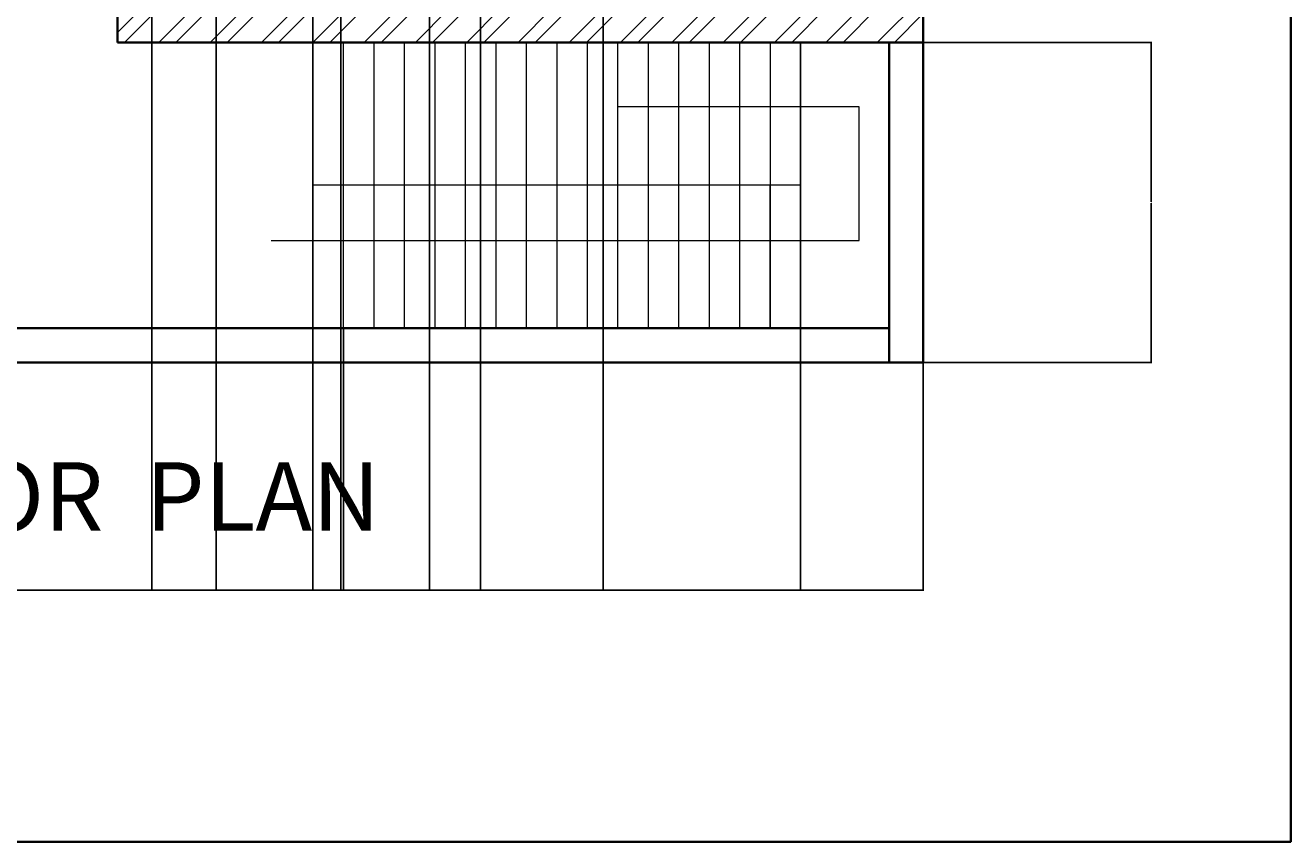
# Model space of a CAD drawing. Units: inches. Extents: x 2552 to 3217, y 1417 to 2737.
# Tile 4 of 25: x 2885 to 3217, y 1417 to 1631. Entities that reach past the tile are written whole.
import ezdxf

# ---------------------------------------------------------------- set-up
doc = ezdxf.new("R2010")
doc.units = ezdxf.units.IN
for name, color, linetype, lineweight in [('A-ANNO-DIMS', 2, 'Continuous', 18), ('A-ANNO-TEXT', 7, 'Continuous', 25), ('A-ANNO-TTLB', 7, 'Continuous', 35), ('A-FLOR-STRS', 140, 'Continuous', 20), ('A-WALL', 7, 'Continuous', 35), ('A-WALL-PATT', 217, 'Continuous', 13)]:
    doc.layers.add(name, color=color, linetype=linetype, lineweight=lineweight)
doc.styles.get("Standard").update_dxf_attribs({"font": 'arial.ttf'})
doc.dimstyles.get("Standard").update_dxf_attribs({"dimtxt": 0.18, "dimasz": 0.18, "dimexe": 0.18, "dimexo": 0.0625, "dimgap": 0.09, "dimtad": 0, "dimtih": 1, "dimtoh": 1, "dimdec": 4, "dimzin": 0, "dimdsep": 46, "dimtxsty": 'Standard', "dimcen": 0.09, "dimadec": 0, "dimazin": 0, "dimtfac": 1, "dimtdec": 4, "dimtofl": 0, "dimtmove": 0, "dimatfit": 3, "dimfxl": 1, "dimtolj": 1, "dimtzin": 0, "dimarcsym": 0})

# ---------------------------------------------------------------- blocks, each defined once
blk = doc.blocks.new('*D49')
at = {"layer": 'A-ANNO-DIMS', "color": 0, "lineweight": -2, "transparency": 16777216}
for p, q in [((2637.35, 1542.45), (2637.35, 1482.53)), ((3120.35, 1542.45), (3120.35, 1482.53)), ((2637.53, 1482.71), (2878.56, 1482.71)), ((3120.17, 1482.71), (2879.15, 1482.71))]:
    blk.add_line(p, q, dxfattribs=at)
at = {"layer": 'A-ANNO-DIMS', "color": 0, "transparency": 16777216}
for points in [[(2637.53, 1482.74), (2637.53, 1482.68), (2637.35, 1482.71)], [(3120.17, 1482.74), (3120.17, 1482.68), (3120.35, 1482.71)]]:
    blk.add_solid(points, dxfattribs=at)
at = {"layer": 'Defpoints', "color": 0, "transparency": 16777216}
for p in [(2637.35, 1542.51), (3120.35, 1542.51), (3120.35, 1482.71)]:
    blk.add_point(p, dxfattribs=at)
at = {"layer": 'A-ANNO-DIMS', "color": 0, "transparency": 16777216, "insert": (2878.85, 1482.71), "char_height": 0.18, "attachment_point": 5}
blk.add_mtext('\\A1;483', dxfattribs=at)
blk = doc.blocks.new('*D53')
at = {"layer": 'A-ANNO-DIMS', "color": 0, "lineweight": -2, "transparency": 16777216}
for p, q in [((3120.42, 1626.51), (3180.33, 1626.51)), ((3180.15, 1626.33), (3180.15, 1584.69)), ((3180.15, 1542.69), (3180.15, 1584.33)), ((3120.42, 1542.51), (3180.33, 1542.51))]:
    blk.add_line(p, q, dxfattribs=at)
at = {"layer": 'A-ANNO-DIMS', "color": 0, "transparency": 16777216}
for points in [[(3180.12, 1626.33), (3180.18, 1626.33), (3180.15, 1626.51)], [(3180.12, 1542.69), (3180.18, 1542.69), (3180.15, 1542.51)]]:
    blk.add_solid(points, dxfattribs=at)
at = {"layer": 'Defpoints', "color": 0, "transparency": 16777216}
for p in [(3120.35, 1626.51), (3180.15, 1626.51), (3120.35, 1542.51)]:
    blk.add_point(p, dxfattribs=at)
at = {"layer": 'A-ANNO-DIMS', "color": 0, "transparency": 16777216, "insert": (3180.15, 1584.51), "char_height": 0.18, "attachment_point": 5}
blk.add_mtext('\\A1;84', dxfattribs=at)
blk = doc.blocks.new('*D56')
at = {"layer": 'A-ANNO-DIMS', "color": 0, "lineweight": -2, "transparency": 16777216}
for p, q in [((2967.49, 2515.95), (2967.49, 1482.53)), ((2990.69, 2515.95), (2990.69, 1482.53)), ((2967.67, 1482.71), (2978.76, 1482.71)), ((2990.51, 1482.71), (2979.41, 1482.71))]:
    blk.add_line(p, q, dxfattribs=at)
at = {"layer": 'A-ANNO-DIMS', "color": 0, "transparency": 16777216}
for points in [[(2967.67, 1482.74), (2967.67, 1482.68), (2967.49, 1482.71)], [(2990.51, 1482.74), (2990.51, 1482.68), (2990.69, 1482.71)]]:
    blk.add_solid(points, dxfattribs=at)
at = {"layer": 'Defpoints', "color": 0, "transparency": 16777216}
for p in [(2967.49, 2516.01), (2990.69, 2516.01), (2990.69, 1482.71)]:
    blk.add_point(p, dxfattribs=at)
at = {"layer": 'A-ANNO-DIMS', "color": 0, "transparency": 16777216, "insert": (2979.09, 1482.71), "char_height": 0.18, "attachment_point": 5}
blk.add_mtext('\\A1;23.2', dxfattribs=at)
blk = doc.blocks.new('*D57')
at = {"layer": 'A-ANNO-DIMS', "color": 0, "lineweight": -2, "transparency": 16777216}
for p, q in [((3004.08, 2515.95), (3004.08, 1482.53)), ((3036.34, 2515.95), (3036.34, 1482.53)), ((3004.26, 1482.71), (3019.75, 1482.71)), ((3036.16, 1482.71), (3020.68, 1482.71))]:
    blk.add_line(p, q, dxfattribs=at)
at = {"layer": 'A-ANNO-DIMS', "color": 0, "transparency": 16777216}
for points in [[(3004.26, 1482.74), (3004.26, 1482.68), (3004.08, 1482.71)], [(3036.16, 1482.74), (3036.16, 1482.68), (3036.34, 1482.71)]]:
    blk.add_solid(points, dxfattribs=at)
at = {"layer": 'Defpoints', "color": 0, "transparency": 16777216}
for p in [(3004.08, 2516.01), (3036.34, 2516.01), (3036.34, 1482.71)]:
    blk.add_point(p, dxfattribs=at)
at = {"layer": 'A-ANNO-DIMS', "color": 0, "transparency": 16777216, "insert": (3020.21, 1482.71), "char_height": 0.18, "attachment_point": 5}
blk.add_mtext('\\A1;32.255', dxfattribs=at)
blk = doc.blocks.new('*D62')
at = {"layer": 'A-ANNO-DIMS', "color": 0, "lineweight": -2, "transparency": 16777216}
for p, q in [((2960.11, 1626.45), (2960.11, 1482.53)), ((3088.11, 1626.45), (3088.11, 1482.53)), ((2960.29, 1482.71), (3023.83, 1482.71)), ((3087.93, 1482.71), (3024.39, 1482.71))]:
    blk.add_line(p, q, dxfattribs=at)
at = {"layer": 'A-ANNO-DIMS', "color": 0, "transparency": 16777216}
for points in [[(2960.29, 1482.74), (2960.29, 1482.68), (2960.11, 1482.71)], [(3087.93, 1482.74), (3087.93, 1482.68), (3088.11, 1482.71)]]:
    blk.add_solid(points, dxfattribs=at)
at = {"layer": 'Defpoints', "color": 0, "transparency": 16777216}
for p in [(2960.11, 1626.51), (3088.11, 1626.51), (3088.11, 1482.71)]:
    blk.add_point(p, dxfattribs=at)
at = {"layer": 'A-ANNO-DIMS', "color": 0, "transparency": 16777216, "insert": (3024.11, 1482.71), "char_height": 0.18, "attachment_point": 5}
blk.add_mtext('\\A1;128', dxfattribs=at)
blk = doc.blocks.new('*D63')
at = {"layer": 'A-ANNO-DIMS', "color": 0, "lineweight": -2, "transparency": 16777216}
for p, q in [((2960.11, 1551.45), (2960.11, 1482.53)), ((2968.11, 1551.45), (2968.11, 1482.53)), ((2960.29, 1482.71), (2963.96, 1482.71)), ((2967.93, 1482.71), (2964.26, 1482.71))]:
    blk.add_line(p, q, dxfattribs=at)
at = {"layer": 'A-ANNO-DIMS', "color": 0, "transparency": 16777216}
for points in [[(2960.29, 1482.74), (2960.29, 1482.68), (2960.11, 1482.71)], [(2967.93, 1482.74), (2967.93, 1482.68), (2968.11, 1482.71)]]:
    blk.add_solid(points, dxfattribs=at)
at = {"layer": 'Defpoints', "color": 0, "transparency": 16777216}
for p in [(2960.11, 1551.51), (2968.11, 1551.51), (2968.11, 1482.71)]:
    blk.add_point(p, dxfattribs=at)
at = {"layer": 'A-ANNO-DIMS', "color": 0, "transparency": 16777216, "insert": (2964.11, 1482.71), "char_height": 0.18, "attachment_point": 5}
blk.add_mtext('\\A1;8', dxfattribs=at)
blk = doc.blocks.new('*D64')
at = {"layer": 'A-ANNO-DIMS', "color": 0, "lineweight": -2, "transparency": 16777216}
for p, q in [((2646.35, 1551.58), (2646.35, 2709.49)), ((2646.53, 2709.31), (2802.77, 2709.31)), ((2959.93, 2709.31), (2803.69, 2709.31)), ((2960.11, 1551.58), (2960.11, 2709.49))]:
    blk.add_line(p, q, dxfattribs=at)
at = {"layer": 'A-ANNO-DIMS', "color": 0, "transparency": 16777216}
for points in [[(2646.53, 2709.34), (2646.53, 2709.28), (2646.35, 2709.31)], [(2959.93, 2709.34), (2959.93, 2709.28), (2960.11, 2709.31)]]:
    blk.add_solid(points, dxfattribs=at)
at = {"layer": 'Defpoints', "color": 0, "transparency": 16777216}
for p in [(2960.11, 2709.31), (2646.35, 1551.51), (2960.11, 1551.51)]:
    blk.add_point(p, dxfattribs=at)
at = {"layer": 'A-ANNO-DIMS', "color": 0, "transparency": 16777216, "insert": (2803.23, 2709.31), "char_height": 0.18, "attachment_point": 5}
blk.add_mtext('\\A1;313.76', dxfattribs=at)
blk = doc.blocks.new('*D67')
at = {"layer": 'A-ANNO-DIMS', "color": 0, "lineweight": -2, "transparency": 16777216}
for p, q in [((2917.85, 2640.45), (2917.85, 1482.53)), ((2934.77, 2624.73), (2934.77, 1482.53)), ((2918.03, 1482.71), (2925.86, 1482.71)), ((2934.59, 1482.71), (2926.76, 1482.71))]:
    blk.add_line(p, q, dxfattribs=at)
at = {"layer": 'A-ANNO-DIMS', "color": 0, "transparency": 16777216}
for points in [[(2918.03, 1482.74), (2918.03, 1482.68), (2917.85, 1482.71)], [(2934.59, 1482.74), (2934.59, 1482.68), (2934.77, 1482.71)]]:
    blk.add_solid(points, dxfattribs=at)
at = {"layer": 'Defpoints', "color": 0, "transparency": 16777216}
for p in [(2917.85, 2640.51), (2934.77, 2624.79), (2934.77, 1482.71)]:
    blk.add_point(p, dxfattribs=at)
at = {"layer": 'A-ANNO-DIMS', "color": 0, "transparency": 16777216, "insert": (2926.31, 1482.71), "char_height": 0.18, "attachment_point": 5}
blk.add_mtext('\\A1;16.912', dxfattribs=at)

msp = doc.modelspace()

# ---------------------------------------------------------------- hatches: boundary and pattern name
at = {"layer": 'A-WALL-PATT'}
h = msp.add_hatch(dxfattribs=at)
h.set_pattern_fill('ANSI32', color=256)
h.paths.add_polyline_path([(2756.676, 2649.5125), (2637.3535, 2649.5125), (2637.3535, 2617.9626), (2641.8535, 2617.9626), (2646.3535, 2617.9626), (2646.3535, 2640.5125), (2724.3535, 2640.5125), (2724.3535, 2520.5125), (2720.299, 2520.5125), (2720.299, 2516.0125), (2733.4075, 2516.0125), (2733.4075, 2518.2213), (2733.4075, 2520.5125), (2728.8535, 2520.5125), (2728.8535, 2640.5125), (2756.676, 2640.5125)])
h.paths.add_polyline_path([(2848.8535, 2649.5125), (2804.676, 2649.5125), (2804.676, 2640.5125), (2839.8535, 2640.5125), (2839.8535, 2598.3517), (2848.8535, 2598.3517)])
h.paths.add_polyline_path([(2646.3535, 2516.0125), (2697.9593, 2516.0125), (2697.9593, 2518.2625), (2697.9593, 2520.5125), (2646.3535, 2520.5125), (2646.3535, 2581.9626), (2637.3535, 2581.9626), (2637.3535, 2364.3298), (2646.3535, 2364.3298), (2646.3535, 2387.0125), (2724.3535, 2387.0125), (2724.3535, 2267.0125), (2721.0443, 2267.0125), (2721.0443, 2262.5125), (2733.7854, 2262.5125), (2733.7854, 2264.7625), (2733.7854, 2267.0125), (2728.8535, 2267.0125), (2728.8535, 2387.0125), (2839.8535, 2387.0125), (2839.8535, 2363.8387), (2848.8535, 2363.8387), (2848.8535, 2403.7415), (2844.3535, 2403.7415), (2839.8535, 2403.7415), (2839.8535, 2396.0125), (2646.3535, 2396.0125)])
h.paths.add_polyline_path([(2848.8535, 2550.3517), (2844.3535, 2550.3517), (2839.8535, 2550.3517), (2839.8535, 2520.5125), (2801.9195, 2520.5125), (2801.9195, 2518.2625), (2801.9195, 2516.0125), (2839.8535, 2516.0125), (2839.8535, 2507.5813), (2848.8535, 2507.5813)], flags=17)
h.paths.add_polyline_path([(2848.8535, 2483.5813), (2844.3535, 2483.5813), (2839.8535, 2483.5813), (2839.8535, 2468.0125), (2773.8535, 2468.0125), (2773.8535, 2516.0125), (2778.1336, 2516.0125), (2778.1336, 2520.5125), (2766.696, 2520.5125), (2766.696, 2518.2625), (2766.696, 2516.0125), (2769.3535, 2516.0125), (2769.3535, 2463.5125), (2839.8535, 2463.5125), (2839.8535, 2431.0782), (2848.8535, 2431.0782)], flags=17)
h.paths.add_polyline_path([(2917.8535, 2569.2764), (2913.3535, 2569.2764), (2908.8535, 2569.2764), (2908.8535, 2433.001), (2917.8535, 2433.001), (2917.8535, 2516.0125), (2967.486, 2516.0125), (2967.486, 2520.5125), (2917.8535, 2520.5125)])
h.paths.add_polyline_path([(3000.3535, 2640.5125), (2995.8535, 2640.5125), (2995.8535, 2520.5125), (2990.688, 2520.5125), (2990.688, 2516.0125), (3004.0844, 2516.0125), (3004.0844, 2518.2625), (3004.0844, 2520.5125), (3000.3535, 2520.5125)])
h.paths.add_polyline_path([(3120.3535, 2561.3689), (3115.8535, 2561.3689), (3111.3535, 2561.3689), (3111.3535, 2520.5125), (3070.9814, 2520.5125), (3070.9814, 2518.2625), (3070.9814, 2516.0125), (3111.3535, 2516.0125), (3111.3535, 2505.1841), (3120.3535, 2505.1841)])
h.paths.add_polyline_path([(3120.3535, 2481.1841), (3115.8535, 2481.1841), (3111.3535, 2481.1841), (3111.3535, 2468.0125), (3045.3535, 2468.0125), (3045.3535, 2516.0125), (3048.9787, 2516.0125), (3048.9787, 2520.5125), (3036.3395, 2520.5125), (3036.3395, 2516.0125), (3040.8535, 2516.0125), (3040.8535, 2463.5125), (3111.3535, 2463.5125), (3111.3535, 2396.0125), (2917.8535, 2396.0125), (2917.8535, 2403.4124), (2913.3535, 2403.4124), (2908.8535, 2403.4124), (2908.8535, 2182.5756), (2917.8535, 2182.5756), (2917.8535, 2262.5125), (2968.001, 2262.5125), (2968.001, 2264.7625), (2968.001, 2267.0125), (2917.8535, 2267.0125), (2917.8535, 2387.0125), (3111.3535, 2387.0125), (3111.3535, 2352.2435), (3120.3535, 2352.2435)])
h.paths.add_polyline_path([(3120.3535, 2304.2435), (3115.8535, 2304.2435), (3111.3535, 2304.2435), (3111.3535, 2267.0125), (3073.8616, 2267.0125), (3073.8616, 2264.7625), (3073.8616, 2262.5125), (3111.3535, 2262.5125), (3111.3535, 2252.376), (3120.3535, 2252.376)], flags=17)
h.paths.add_polyline_path([(3120.3535, 2228.376), (3115.8535, 2228.376), (3111.3535, 2228.376), (3111.3535, 2214.5125), (3045.3535, 2214.5125), (3045.3535, 2262.5125), (3049.3096, 2262.5125), (3049.3096, 2267.0125), (3035.0125, 2267.0125), (3035.0125, 2262.5125), (3040.8535, 2262.5125), (3040.8535, 2210.0125), (3111.3535, 2210.0125), (3111.3535, 2142.5125), (2917.8535, 2142.5125), (2917.8535, 2150.2408), (2913.3535, 2150.2408), (2908.8535, 2150.2408), (2908.8535, 1924.9905), (2917.8535, 1924.9905), (2917.8535, 2009.0125), (2971.959, 2009.0125), (2971.959, 2011.2625), (2971.959, 2013.5125), (2917.8535, 2013.5125), (2917.8535, 2133.5125), (2995.8535, 2133.5125), (2995.8535, 2013.5125), (2992.1797, 2013.5125), (2992.1797, 2009.0125), (3004.3344, 2009.0125), (3004.3344, 2011.2625), (3004.3344, 2013.5125), (3000.3535, 2013.5125), (3000.3535, 2133.5125), (3111.3535, 2133.5125), (3111.3535, 2115.0291), (3120.3535, 2115.0291)])
h.paths.add_polyline_path([(3000.3535, 2387.0125), (2995.8535, 2387.0125), (2995.8535, 2267.0125), (2991.3326, 2267.0125), (2991.3326, 2262.5125), (3004.1044, 2262.5125), (3004.1044, 2264.7625), (3004.1044, 2267.0125), (3000.3535, 2267.0125)], flags=17)
h.paths.add_polyline_path([(3120.3535, 1973.2388), (3115.8535, 1973.2388), (3111.3535, 1973.2388), (3111.3535, 1961.0125), (3045.3535, 1961.0125), (3045.3535, 2009.0125), (3048.9101, 2009.0125), (3048.9101, 2013.5125), (3037.105, 2013.5125), (3037.105, 2011.2625), (3037.105, 2009.0125), (3040.8535, 2009.0125), (3040.8535, 1956.5125), (3111.3535, 1956.5125), (3111.3535, 1889.0125), (2917.8535, 1889.0125), (2917.8535, 1895.7215), (2913.3535, 1895.7215), (2908.8535, 1895.7215), (2908.8535, 1844.2217), (2917.8535, 1844.2217), (2917.8535, 1880.0125), (3111.3535, 1880.0125), (3111.3535, 1846.9541), (3120.3535, 1846.9541)])
h.paths.add_polyline_path([(3120.3535, 2067.0291), (3111.3535, 2067.0291), (3111.3535, 2013.5125), (3071.3001, 2013.5125), (3071.3001, 2009.0125), (3111.3535, 2009.0125), (3111.3535, 1997.2388), (3120.3535, 1997.2388)], flags=0)
h.paths.add_polyline_path([(3120.3535, 1798.9541), (3115.8535, 1798.9541), (3111.3535, 1798.9541), (3111.3535, 1760.0125), (3071.2497, 1760.0125), (3071.2497, 1757.7625), (3071.2497, 1755.5125), (3111.3535, 1755.5125), (3111.3535, 1746.162), (3120.3535, 1746.2478)])
h.paths.add_polyline_path([(3120.3535, 1722.2049), (3111.3535, 1722.2049), (3111.3535, 1707.5125), (3045.3535, 1707.5125), (3045.3535, 1755.5125), (3048.6624, 1755.5125), (3048.6624, 1760.0125), (3035.3703, 1760.0125), (3035.3703, 1755.5125), (3040.8535, 1755.5125), (3040.8535, 1703.0125), (3111.3535, 1703.0125), (3111.3535, 1635.5125), (2917.8535, 1635.5125), (2917.8535, 1643.1366), (2913.3535, 1643.1366), (2908.8535, 1643.1366), (2908.8535, 1626.5125), (3120.3535, 1626.5125)])
h.paths.add_polyline_path([(2917.8535, 1755.5125), (2973.2287, 1755.5125), (2973.2287, 1757.7625), (2973.2287, 1760.0125), (2917.8535, 1760.0125), (2917.8535, 1808.2217), (2913.3535, 1808.2217), (2908.8535, 1808.2217), (2908.8535, 1676.1665), (2917.8535, 1676.1665)])
h.paths.add_polyline_path([(3000.3535, 1880.0125), (2995.8535, 1880.0125), (2995.8535, 1760.0125), (2992.9329, 1760.0125), (2992.9329, 1755.5125), (3003.8766, 1755.5125), (3003.8766, 1757.7625), (3003.8766, 1760.0125), (3000.3535, 1760.0125)])
h.paths.add_polyline_path([(2848.8535, 1896.6971), (2844.3535, 1896.6971), (2839.8535, 1896.6971), (2839.8535, 1889.0125), (2646.3535, 1889.0125), (2646.3535, 2009.0125), (2700.5253, 2009.0125), (2700.5253, 2011.2625), (2700.5253, 2013.5125), (2646.3535, 2013.5125), (2646.3535, 2053.1812), (2641.8535, 2053.1812), (2637.3535, 2053.1812), (2637.3535, 1836.254), (2646.3535, 1836.254), (2646.3535, 1880.0125), (2724.3535, 1880.0125), (2724.3535, 1760.0125), (2721.2473, 1760.0125), (2721.2473, 1755.5125), (2731.9187, 1755.5125), (2731.9187, 1757.7625), (2731.9187, 1760.0125), (2728.8535, 1760.0125), (2728.8535, 1880.0125), (2839.8535, 1880.0125), (2839.8535, 1840.3813), (2848.8535, 1840.3813)])
h.paths.add_polyline_path([(2848.8535, 1792.3813), (2844.3535, 1792.3813), (2839.8535, 1792.3813), (2839.8535, 1760.0125), (2797.8845, 1760.0125), (2797.8845, 1755.5125), (2839.8535, 1755.5125), (2839.8535, 1743.3688), (2844.3535, 1743.3688), (2848.8535, 1743.3688)], flags=0)
h.paths.add_polyline_path([(2848.8535, 1719.3688), (2844.3535, 1719.3688), (2839.8535, 1719.3688), (2839.8535, 1707.5125), (2773.8535, 1707.5125), (2773.8535, 1755.5125), (2777.716, 1755.5125), (2777.716, 1760.0125), (2760.9247, 1760.0125), (2760.9247, 1757.9721), (2760.9247, 1755.5125), (2769.3535, 1755.5125), (2769.3535, 1703.0125), (2839.8535, 1703.0125), (2839.8535, 1673.0277), (2848.8535, 1672.9407)], flags=0)
h.paths.add_polyline_path([(2646.3535, 1755.5125), (2702.9171, 1755.5125), (2702.9171, 1757.7625), (2702.9171, 1760.0125), (2646.3535, 1760.0125), (2646.3535, 1800.254), (2641.8535, 1800.254), (2637.3535, 1800.254), (2637.3535, 1626.5125), (2848.8535, 1626.5125), (2848.8535, 1643.1187), (2844.3535, 1643.1187), (2839.8535, 1643.1187), (2839.8535, 1635.5125), (2646.3535, 1635.5125)])
h.paths.add_polyline_path([(2848.8535, 2148.8427), (2844.3535, 2148.8427), (2839.8535, 2148.8427), (2839.8535, 2142.5125), (2646.3535, 2142.5125), (2646.3535, 2262.5125), (2701.3562, 2262.5125), (2701.3562, 2264.7625), (2701.3562, 2267.0125), (2646.3535, 2267.0125), (2646.3535, 2328.3298), (2637.3535, 2328.3298), (2637.3535, 2089.1812), (2646.3535, 2089.1812), (2646.3535, 2133.5125), (2839.8535, 2133.5125), (2839.8535, 2097.5966), (2848.8535, 2097.5966)])
h.paths.add_polyline_path([(2728.8535, 2133.5125), (2724.3535, 2133.5125), (2724.3535, 2013.5125), (2719.6039, 2013.5125), (2719.6039, 2009.0125), (2732.5784, 2009.0125), (2732.5784, 2011.2625), (2732.5784, 2013.5125), (2728.8535, 2013.5125)])
h.paths.add_polyline_path([(2848.8535, 1970.0557), (2844.3535, 1970.0557), (2839.8535, 1970.0557), (2839.8535, 1961.0125), (2773.8535, 1961.0125), (2773.8535, 2009.0125), (2777.3388, 2009.0125), (2777.3388, 2013.5125), (2764.7681, 2013.5125), (2764.7681, 2009.0125), (2769.3535, 2009.0125), (2769.3535, 1956.5125), (2839.8535, 1956.5125), (2839.8535, 1924.7199), (2848.8535, 1924.7199)], flags=17)
h.paths.add_polyline_path([(2848.8535, 2049.5966), (2844.3535, 2049.5966), (2839.8535, 2049.5966), (2839.8535, 2013.5125), (2798.198, 2013.5125), (2798.198, 2011.2625), (2798.198, 2009.0125), (2839.8535, 2009.0125), (2839.8535, 1994.0557), (2848.8535, 1994.0557)], flags=17)
h.paths.add_polyline_path([(2848.8535, 2315.8387), (2839.8535, 2315.8387), (2839.8535, 2267.0125), (2799.3375, 2267.0125), (2799.3375, 2264.7625), (2799.3375, 2262.5125), (2839.8535, 2262.5125), (2839.8535, 2253.2843), (2848.8535, 2253.2843)], flags=17)
h.paths.add_polyline_path([(2848.8535, 2229.2843), (2839.8535, 2229.2843), (2839.8535, 2177.6936), (2848.8535, 2177.6936)], flags=17)
h.paths.add_polyline_path([(2839.8535, 2214.5125), (2773.8535, 2214.5125), (2773.8535, 2262.5125), (2777.6984, 2262.5125), (2777.6984, 2267.0125), (2763.8226, 2267.0125), (2763.8226, 2262.5125), (2769.3535, 2262.5125), (2769.3535, 2210.0125), (2839.8535, 2210.0125)], flags=17)
h.paths.add_polyline_path([(3050.32, 2520.2817), (3088.9114, 2520.2817), (3088.9114, 2538.939), (3050.32, 2538.939)], flags=9)

# ---------------------------------------------------------------- linework, layer by layer
at = {"layer": 'A-ANNO-TTLB'}
msp.add_lwpolyline([(2552.473, 2736.5692), (3216.7862, 2736.5692), (3216.7862, 1416.6914), (2552.473, 1416.6914)], close=True, dxfattribs=at)
at = {"layer": 'A-FLOR-STRS'}
for p, q in [((2960.1089, 1626.5125), (2960.1089, 1551.5125)), ((2968.1089, 1626.5125), (2968.1089, 1551.5125)), ((2976.1089, 1626.5125), (2976.1089, 1551.5125)), ((2984.1089, 1626.5125), (2984.1089, 1551.5125)), ((2992.1089, 1626.5125), (2992.1089, 1551.5125)), ((3000.1089, 1626.5125), (3000.1089, 1551.5125)), ((3008.1089, 1626.5125), (3008.1089, 1551.5125)), ((3016.1089, 1626.5125), (3016.1089, 1551.5125)), ((3024.1089, 1626.5125), (3024.1089, 1551.5125)), ((3032.1089, 1626.5125), (3032.1089, 1551.5125)), ((3040.1089, 1626.5125), (3040.1089, 1551.5125)), ((3048.1089, 1626.5125), (3048.1089, 1551.5125)), ((3056.1089, 1626.5125), (3056.1089, 1551.5125)), ((3064.1089, 1626.5125), (3064.1089, 1551.5125)), ((3072.1089, 1626.5125), (3072.1089, 1551.5125)), ((3080.1089, 1626.5125), (3080.1089, 1551.5125)), ((3088.1089, 1626.5125), (3088.1089, 1551.5125)), ((3103.5182, 1609.6265), (3040.1089, 1609.6265)), ((3103.5182, 1574.534), (3103.5182, 1609.6265)), ((3088.1089, 1589.0125), (2960.1089, 1589.0125)), ((3080.1089, 1551.5125), (3080.1089, 1589.0125)), ((3088.1089, 1551.5125), (3088.1089, 1589.0125)), ((2949.1274, 1574.534), (3103.5182, 1574.534))]:
    msp.add_line(p, q, dxfattribs=at)
at = {"layer": 'A-WALL'}
for p, q in [((3120.3535, 1722.2049), (3120.3535, 1626.5125)), ((2908.8535, 1643.1366), (2908.8535, 1626.5125)), ((2908.8535, 1626.5125), (3120.3535, 1626.5125)), ((3111.3535, 1626.5125), (3111.3535, 1542.5125)), ((3120.3535, 1626.5125), (3120.3535, 1566.5125)), ((3120.3535, 1566.5125), (3120.3535, 1542.5125)), ((3111.3535, 1551.5125), (2646.3535, 1551.5125)), ((3111.3535, 1547.0125), (3111.3535, 1551.5125)), ((3111.3535, 1542.5125), (3111.3535, 1547.0125)), ((2938.5018, 1542.5125), (2637.3535, 1542.5125)), ((3120.3535, 1542.5125), (2938.5018, 1542.5125))]:
    msp.add_line(p, q, dxfattribs=at)

# ---------------------------------------------------------------- texts
at = {"layer": 'A-ANNO-TEXT', "insert": (2749.5428, 1516.3052), "char_height": 18, "attachment_point": 1}
msp.add_mtext_dynamic_manual_height_columns('{FIRST  FLOOR  PLAN}', width=366.4635, gutter_width=12.5, heights=[0], dxfattribs=at)

# ---------------------------------------------------------------- dimensions: what is measured, and where the dimension line sits
at = {"layer": 'A-ANNO-DIMS'}
for base, p1, p2, override, picture, middle in [((2960.1089, 2709.3125), (2646.3535, 1551.5125), (2960.1089, 1551.5125), {"dimdec": 2, "dimlfac": 1, "dimrnd": 0, "dimzin": 0, "dimdsep": 46, "dimlunit": 2}, '*D64', (2803.2312, 2709.3125)), ((2934.7654, 1482.7125), (2917.8535, 2640.5125), (2934.7654, 2624.7942), {"dimdec": 3, "dimlfac": 1, "dimrnd": 0, "dimzin": 0, "dimdsep": 46, "dimlunit": 2}, '*D67', (2926.3094, 1482.7125)), ((2990.688, 1482.7125), (2967.486, 2516.0125), (2990.688, 2516.0125), {"dimdec": 1, "dimlfac": 1, "dimrnd": 0, "dimzin": 0, "dimdsep": 46, "dimlunit": 2}, '*D56', (2979.087, 1482.7125)), ((3036.3395, 1482.7125), (3004.0844, 2516.0125), (3036.3395, 2516.0125), {"dimdec": 3, "dimlfac": 1, "dimrnd": 0, "dimzin": 0, "dimdsep": 46, "dimlunit": 2}, '*D57', (3020.212, 1482.7125)), ((3088.1089, 1482.7125), (2960.1089, 1626.5125), (3088.1089, 1626.5125), {"dimdec": 0, "dimlfac": 1, "dimrnd": 0, "dimzin": 0, "dimdsep": 46, "dimlunit": 2}, '*D62', (3024.1089, 1482.7125)), ((2968.1089, 1482.7125), (2960.1089, 1551.5125), (2968.1089, 1551.5125), {"dimdec": 0, "dimlfac": 1, "dimrnd": 0, "dimzin": 0, "dimdsep": 46, "dimlunit": 2}, '*D63', (2964.1089, 1482.7125)), ((3120.3535, 1482.7125), (2637.3535, 1542.5125), (3120.3535, 1542.5125), {"dimdec": 0, "dimlfac": 1, "dimrnd": 0, "dimzin": 0, "dimdsep": 46, "dimlunit": 2}, '*D49', (2878.8535, 1482.7125))]:
    dim = msp.add_linear_dim(base=base, p1=p1, p2=p2, dimstyle='Standard', override=override, dxfattribs=at)
    dim.commit()
    dim.dimension.update_dxf_attribs({"geometry": picture, "text_midpoint": middle})
dim = msp.add_linear_dim(base=(3180.1535, 1626.5125), p1=(3120.3535, 1542.5125), p2=(3120.3535, 1626.5125), angle=90, dimstyle='Standard', override={"dimdec": 0, "dimlfac": 1, "dimrnd": 0, "dimzin": 0, "dimdsep": 46, "dimlunit": 2}, dxfattribs=at)
dim.commit()
dim.dimension.update_dxf_attribs({"geometry": '*D53', "text_midpoint": (3180.1535, 1584.5125)})

doc.saveas('drawing.dxf')
